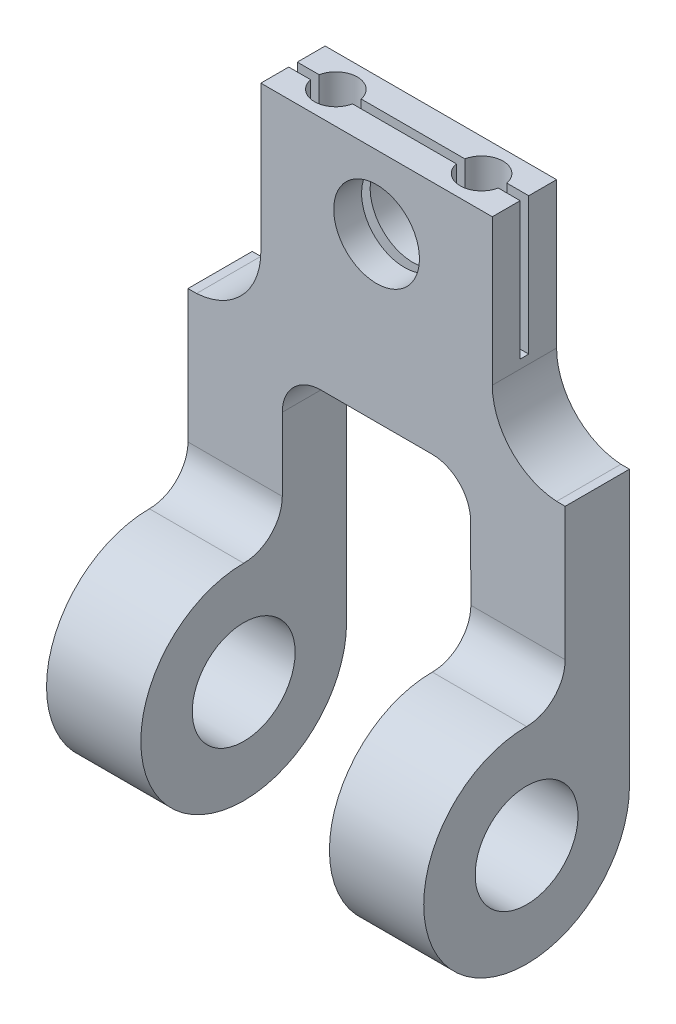
ISO-10303-21;
HEADER;
FILE_DESCRIPTION(('STEP AP214'),'2;1');
FILE_NAME('part.step','',(''),(''),'','','');
FILE_SCHEMA(('AUTOMOTIVE_DESIGN { 1 0 10303 214 1 1 1 1 }'));
ENDSEC;
DATA;
#1=APPLICATION_CONTEXT('core data for automotive mechanical design processes');
#2=APPLICATION_PROTOCOL_DEFINITION('international standard','automotive_design',2000,#1);
#3=PRODUCT_CONTEXT('',#1,'mechanical');
#4=PRODUCT('Part','Part','',(#3));
#5=PRODUCT_RELATED_PRODUCT_CATEGORY('part','',(#4));
#6=PRODUCT_DEFINITION_FORMATION('','',#4);
#7=PRODUCT_DEFINITION_CONTEXT('part definition',#1,'design');
#8=PRODUCT_DEFINITION('design','',#6,#7);
#9=PRODUCT_DEFINITION_SHAPE('','',#8);
#10=(LENGTH_UNIT() NAMED_UNIT(*) SI_UNIT(.MILLI.,.METRE.));
#11=(NAMED_UNIT(*) PLANE_ANGLE_UNIT() SI_UNIT($,.RADIAN.));
#12=(NAMED_UNIT(*) SI_UNIT($,.STERADIAN.) SOLID_ANGLE_UNIT());
#13=UNCERTAINTY_MEASURE_WITH_UNIT(LENGTH_MEASURE(1.E-05),#10,'distance_accuracy_value','');
#14=(GEOMETRIC_REPRESENTATION_CONTEXT(3) GLOBAL_UNCERTAINTY_ASSIGNED_CONTEXT((#13)) GLOBAL_UNIT_ASSIGNED_CONTEXT((#10,
#11,#12)) REPRESENTATION_CONTEXT('',''));
#15=CARTESIAN_POINT('',(0.,0.,0.));
#16=DIRECTION('',(0.,0.,1.));
#17=DIRECTION('',(1.,0.,0.));
#18=AXIS2_PLACEMENT_3D('',#15,#16,#17);
#19=CARTESIAN_POINT('',(88.,114.000000000021,-17.5));
#20=DIRECTION('',(0.,0.,-1.));
#21=DIRECTION('',(0.,1.,0.));
#22=AXIS2_PLACEMENT_3D('',#19,#20,#21);
#23=PLANE('',#22);
#24=DIRECTION('',(-1.,0.,0.));
#25=VECTOR('',#24,1.);
#26=CARTESIAN_POINT('',(88.,82.0000000000214,-17.5));
#27=LINE('',#26,#25);
#28=CARTESIAN_POINT('',(22.1010205144336,82.0000000000214,-17.5));
#29=VERTEX_POINT('',#28);
#30=CARTESIAN_POINT('',(17.,82.0000000000214,-17.5));
#31=VERTEX_POINT('',#30);
#32=EDGE_CURVE('E292',#29,#31,#27,.T.);
#33=ORIENTED_EDGE('',*,*,#32,.F.);
#34=DIRECTION('',(0.,1.,0.));
#35=VECTOR('',#34,1.);
#36=CARTESIAN_POINT('',(22.1010205144336,82.0000000000214,-17.5));
#37=LINE('',#36,#35);
#38=CARTESIAN_POINT('',(22.1010205144336,114.000000000021,-17.5));
#39=VERTEX_POINT('',#38);
#40=EDGE_CURVE('E341',#29,#39,#37,.T.);
#41=ORIENTED_EDGE('',*,*,#40,.T.);
#42=DIRECTION('',(-1.,0.,0.));
#43=VECTOR('',#42,1.);
#44=CARTESIAN_POINT('',(88.,114.000000000021,-17.5));
#45=LINE('',#44,#43);
#46=CARTESIAN_POINT('',(17.,114.000000000021,-17.5));
#47=VERTEX_POINT('',#46);
#48=EDGE_CURVE('E269',#39,#47,#45,.T.);
#49=ORIENTED_EDGE('',*,*,#48,.T.);
#50=DIRECTION('',(0.,-1.,0.));
#51=VECTOR('',#50,1.);
#52=CARTESIAN_POINT('',(17.,114.000000000021,-17.5));
#53=LINE('',#52,#51);
#54=EDGE_CURVE('E301',#47,#31,#53,.T.);
#55=ORIENTED_EDGE('',*,*,#54,.T.);
#56=EDGE_LOOP('',(#33,#41,#49,#55));
#57=FACE_BOUND('',#56,.T.);
#58=ADVANCED_FACE('F50',(#57),#23,.F.);
#59=CARTESIAN_POINT('',(44.,97.0000000000214,-17.5));
#60=DIRECTION('',(0.,0.,-1.));
#61=DIRECTION('',(0.,1.,0.));
#62=AXIS2_PLACEMENT_3D('',#59,#60,#61);
#63=CIRCLE('',#62,10.);
#64=CARTESIAN_POINT('',(44.,107.000000000021,-17.5));
#65=VERTEX_POINT('',#64);
#66=EDGE_CURVE('E601',#65,#65,#63,.F.);
#67=ORIENTED_EDGE('',*,*,#66,.F.);
#68=EDGE_LOOP('',(#67));
#69=FACE_BOUND('',#68,.T.);
#70=CARTESIAN_POINT('',(56.1010205144336,114.000000000021,-17.5));
#71=VERTEX_POINT('',#70);
#72=CARTESIAN_POINT('',(31.8989794855664,114.000000000021,-17.5));
#73=VERTEX_POINT('',#72);
#74=EDGE_CURVE('E273',#71,#73,#45,.T.);
#75=ORIENTED_EDGE('',*,*,#74,.T.);
#76=DIRECTION('',(0.,1.,0.));
#77=VECTOR('',#76,1.);
#78=CARTESIAN_POINT('',(31.8989794855664,82.0000000000214,-17.5));
#79=LINE('',#78,#77);
#80=CARTESIAN_POINT('',(31.8989794855664,82.0000000000214,-17.5));
#81=VERTEX_POINT('',#80);
#82=EDGE_CURVE('E317',#73,#81,#79,.F.);
#83=ORIENTED_EDGE('',*,*,#82,.T.);
#84=CARTESIAN_POINT('',(56.1010205144336,82.0000000000214,-17.5));
#85=VERTEX_POINT('',#84);
#86=EDGE_CURVE('E290',#85,#81,#27,.T.);
#87=ORIENTED_EDGE('',*,*,#86,.F.);
#88=DIRECTION('',(0.,1.,0.));
#89=VECTOR('',#88,1.);
#90=CARTESIAN_POINT('',(56.1010205144336,82.0000000000214,-17.5));
#91=LINE('',#90,#89);
#92=EDGE_CURVE('E319',#85,#71,#91,.T.);
#93=ORIENTED_EDGE('',*,*,#92,.T.);
#94=EDGE_LOOP('',(#75,#83,#87,#93));
#95=FACE_BOUND('',#94,.T.);
#96=ADVANCED_FACE('F320',(#69,#95),#23,.F.);
#97=CARTESIAN_POINT('',(88.,114.000000000021,-15.5));
#98=DIRECTION('',(0.,0.,1.));
#99=DIRECTION('',(0.,-1.,0.));
#100=AXIS2_PLACEMENT_3D('',#97,#98,#99);
#101=PLANE('',#100);
#102=CARTESIAN_POINT('',(44.,97.0000000000214,-15.5));
#103=DIRECTION('',(0.,0.,1.));
#104=DIRECTION('',(0.,-1.,0.));
#105=AXIS2_PLACEMENT_3D('',#102,#103,#104);
#106=CIRCLE('',#105,10.);
#107=CARTESIAN_POINT('',(44.,87.0000000000214,-15.5));
#108=VERTEX_POINT('',#107);
#109=EDGE_CURVE('E305',#108,#108,#106,.F.);
#110=ORIENTED_EDGE('',*,*,#109,.F.);
#111=EDGE_LOOP('',(#110));
#112=FACE_BOUND('',#111,.T.);
#113=DIRECTION('',(-1.,0.,0.));
#114=VECTOR('',#113,1.);
#115=CARTESIAN_POINT('',(88.,82.0000000000214,-15.5));
#116=LINE('',#115,#114);
#117=CARTESIAN_POINT('',(56.1010205144336,82.0000000000214,-15.5));
#118=VERTEX_POINT('',#117);
#119=CARTESIAN_POINT('',(31.8989794855664,82.0000000000214,-15.5));
#120=VERTEX_POINT('',#119);
#121=EDGE_CURVE('E283',#118,#120,#116,.T.);
#122=ORIENTED_EDGE('',*,*,#121,.T.);
#123=DIRECTION('',(0.,1.,0.));
#124=VECTOR('',#123,1.);
#125=CARTESIAN_POINT('',(31.8989794855664,82.0000000000214,-15.5));
#126=LINE('',#125,#124);
#127=CARTESIAN_POINT('',(31.8989794855664,114.000000000021,-15.5));
#128=VERTEX_POINT('',#127);
#129=EDGE_CURVE('E11',#120,#128,#126,.T.);
#130=ORIENTED_EDGE('',*,*,#129,.T.);
#131=DIRECTION('',(-1.,0.,0.));
#132=VECTOR('',#131,1.);
#133=CARTESIAN_POINT('',(88.,114.000000000021,-15.5));
#134=LINE('',#133,#132);
#135=CARTESIAN_POINT('',(56.1010205144336,114.000000000021,-15.5));
#136=VERTEX_POINT('',#135);
#137=EDGE_CURVE('E271',#136,#128,#134,.T.);
#138=ORIENTED_EDGE('',*,*,#137,.F.);
#139=DIRECTION('',(0.,1.,0.));
#140=VECTOR('',#139,1.);
#141=CARTESIAN_POINT('',(56.1010205144336,82.0000000000214,-15.5));
#142=LINE('',#141,#140);
#143=EDGE_CURVE('E252',#136,#118,#142,.F.);
#144=ORIENTED_EDGE('',*,*,#143,.T.);
#145=EDGE_LOOP('',(#122,#130,#138,#144));
#146=FACE_BOUND('',#145,.T.);
#147=ADVANCED_FACE('F352',(#112,#146),#101,.F.);
#148=CARTESIAN_POINT('',(71.,82.0000000000214,-15.5));
#149=VERTEX_POINT('',#148);
#150=CARTESIAN_POINT('',(65.8989794855663,82.0000000000214,-15.5));
#151=VERTEX_POINT('',#150);
#152=EDGE_CURVE('E262',#149,#151,#116,.T.);
#153=ORIENTED_EDGE('',*,*,#152,.T.);
#154=DIRECTION('',(0.,1.,0.));
#155=VECTOR('',#154,1.);
#156=CARTESIAN_POINT('',(65.8989794855663,82.0000000000214,-15.5));
#157=LINE('',#156,#155);
#158=CARTESIAN_POINT('',(65.8989794855663,114.000000000021,-15.5));
#159=VERTEX_POINT('',#158);
#160=EDGE_CURVE('E248',#151,#159,#157,.T.);
#161=ORIENTED_EDGE('',*,*,#160,.T.);
#162=CARTESIAN_POINT('',(71.,114.000000000021,-15.5));
#163=VERTEX_POINT('',#162);
#164=EDGE_CURVE('E265',#163,#159,#134,.T.);
#165=ORIENTED_EDGE('',*,*,#164,.F.);
#166=DIRECTION('',(0.,1.,0.));
#167=VECTOR('',#166,1.);
#168=CARTESIAN_POINT('',(71.,0.,-15.5));
#169=LINE('',#168,#167);
#170=EDGE_CURVE('E309',#149,#163,#169,.T.);
#171=ORIENTED_EDGE('',*,*,#170,.F.);
#172=EDGE_LOOP('',(#153,#161,#165,#171));
#173=FACE_BOUND('',#172,.T.);
#174=ADVANCED_FACE('F257',(#173),#101,.F.);
#175=CARTESIAN_POINT('',(0.,114.000000000021,-24.));
#176=DIRECTION('',(0.,-1.,0.));
#177=DIRECTION('',(0.,0.,-1.));
#178=AXIS2_PLACEMENT_3D('',#175,#176,#177);
#179=PLANE('',#178);
#180=ORIENTED_EDGE('',*,*,#48,.F.);
#181=CARTESIAN_POINT('',(27.,114.000000000021,-16.5));
#182=DIRECTION('',(0.,1.,0.));
#183=DIRECTION('',(0.,0.,1.));
#184=AXIS2_PLACEMENT_3D('',#181,#182,#183);
#185=CIRCLE('',#184,5.);
#186=EDGE_CURVE('E326',#73,#39,#185,.T.);
#187=ORIENTED_EDGE('',*,*,#186,.F.);
#188=ORIENTED_EDGE('',*,*,#74,.F.);
#189=CARTESIAN_POINT('',(61.,114.000000000021,-16.5));
#190=DIRECTION('',(0.,1.,0.));
#191=DIRECTION('',(0.,0.,1.));
#192=AXIS2_PLACEMENT_3D('',#189,#190,#191);
#193=CIRCLE('',#192,5.);
#194=CARTESIAN_POINT('',(65.8989794855663,114.000000000021,-17.5));
#195=VERTEX_POINT('',#194);
#196=EDGE_CURVE('E260',#195,#71,#193,.T.);
#197=ORIENTED_EDGE('',*,*,#196,.F.);
#198=CARTESIAN_POINT('',(71.,114.000000000021,-17.5));
#199=VERTEX_POINT('',#198);
#200=EDGE_CURVE('E277',#199,#195,#45,.T.);
#201=ORIENTED_EDGE('',*,*,#200,.F.);
#202=DIRECTION('',(0.,0.,1.));
#203=VECTOR('',#202,1.);
#204=CARTESIAN_POINT('',(71.,114.000000000021,-24.));
#205=LINE('',#204,#203);
#206=CARTESIAN_POINT('',(71.,114.000000000021,-24.));
#207=VERTEX_POINT('',#206);
#208=EDGE_CURVE('E541',#207,#199,#205,.T.);
#209=ORIENTED_EDGE('',*,*,#208,.F.);
#210=DIRECTION('',(1.,0.,0.));
#211=VECTOR('',#210,1.);
#212=CARTESIAN_POINT('',(0.,114.000000000021,-24.));
#213=LINE('',#212,#211);
#214=CARTESIAN_POINT('',(17.,114.000000000021,-24.));
#215=VERTEX_POINT('',#214);
#216=EDGE_CURVE('E488',#215,#207,#213,.T.);
#217=ORIENTED_EDGE('',*,*,#216,.F.);
#218=DIRECTION('',(0.,0.,1.));
#219=VECTOR('',#218,1.);
#220=CARTESIAN_POINT('',(17.,114.000000000021,-24.));
#221=LINE('',#220,#219);
#222=EDGE_CURVE('E538',#215,#47,#221,.T.);
#223=ORIENTED_EDGE('',*,*,#222,.T.);
#224=EDGE_LOOP('',(#180,#187,#188,#197,#201,#209,#217,#223));
#225=FACE_BOUND('',#224,.T.);
#226=ADVANCED_FACE('F324',(#225),#179,.F.);
#227=CARTESIAN_POINT('',(44.,97.0000000000214,-24.));
#228=DIRECTION('',(0.,0.,1.));
#229=DIRECTION('',(1.,0.,0.));
#230=AXIS2_PLACEMENT_3D('',#227,#228,#229);
#231=CYLINDRICAL_SURFACE('',#230,10.);
#232=ORIENTED_EDGE('',*,*,#66,.T.);
#233=EDGE_LOOP('',(#232));
#234=FACE_BOUND('',#233,.T.);
#235=CARTESIAN_POINT('',(44.,97.0000000000214,-24.));
#236=DIRECTION('',(0.,0.,1.));
#237=DIRECTION('',(1.,0.,0.));
#238=AXIS2_PLACEMENT_3D('',#235,#236,#237);
#239=CIRCLE('',#238,10.);
#240=CARTESIAN_POINT('',(54.,97.0000000000214,-24.));
#241=VERTEX_POINT('',#240);
#242=EDGE_CURVE('E474',#241,#241,#239,.T.);
#243=ORIENTED_EDGE('',*,*,#242,.F.);
#244=EDGE_LOOP('',(#243));
#245=FACE_BOUND('',#244,.T.);
#246=ADVANCED_FACE('F387',(#234,#245),#231,.F.);
#247=CARTESIAN_POINT('',(87.,79.9687194226927,-24.));
#248=DIRECTION('',(0.,0.,1.));
#249=DIRECTION('',(1.,0.,0.));
#250=AXIS2_PLACEMENT_3D('',#247,#248,#249);
#251=CYLINDRICAL_SURFACE('',#250,16.);
#252=DIRECTION('',(0.,0.,1.));
#253=VECTOR('',#252,1.);
#254=CARTESIAN_POINT('',(85.9999999999999,64.0000000000214,-24.));
#255=LINE('',#254,#253);
#256=CARTESIAN_POINT('',(85.9999999999999,64.0000000000214,-24.0000000000009));
#257=VERTEX_POINT('',#256);
#258=CARTESIAN_POINT('',(85.9999999999999,64.0000000000214,-9.00000000001455));
#259=VERTEX_POINT('',#258);
#260=EDGE_CURVE('E506',#257,#259,#255,.T.);
#261=ORIENTED_EDGE('',*,*,#260,.F.);
#262=CARTESIAN_POINT('',(87.,79.9687194226927,-24.));
#263=DIRECTION('',(0.,0.,1.));
#264=DIRECTION('',(1.,0.,0.));
#265=AXIS2_PLACEMENT_3D('',#262,#263,#264);
#266=CIRCLE('',#265,16.);
#267=CARTESIAN_POINT('',(71.,79.9687194226927,-24.));
#268=VERTEX_POINT('',#267);
#269=EDGE_CURVE('E476',#268,#257,#266,.T.);
#270=ORIENTED_EDGE('',*,*,#269,.F.);
#271=DIRECTION('',(0.,0.,1.));
#272=VECTOR('',#271,1.);
#273=CARTESIAN_POINT('',(71.,79.9687194226927,-24.));
#274=LINE('',#273,#272);
#275=CARTESIAN_POINT('',(71.,79.9687194226927,-9.00000000000001));
#276=VERTEX_POINT('',#275);
#277=EDGE_CURVE('E542',#268,#276,#274,.T.);
#278=ORIENTED_EDGE('',*,*,#277,.T.);
#279=CARTESIAN_POINT('',(87.,79.9687194226927,-9.00000000000001));
#280=DIRECTION('',(0.,0.,1.));
#281=DIRECTION('',(1.,0.,0.));
#282=AXIS2_PLACEMENT_3D('',#279,#280,#281);
#283=CIRCLE('',#282,16.);
#284=EDGE_CURVE('E521',#276,#259,#283,.T.);
#285=ORIENTED_EDGE('',*,*,#284,.T.);
#286=EDGE_LOOP('',(#261,#270,#278,#285));
#287=FACE_BOUND('',#286,.T.);
#288=ADVANCED_FACE('F423',(#287),#251,.F.);
#289=CARTESIAN_POINT('',(22.,64.,-24.));
#290=DIRECTION('',(0.,-1.,0.));
#291=DIRECTION('',(0.,0.,-1.));
#292=AXIS2_PLACEMENT_3D('',#289,#290,#291);
#293=PLANE('',#292);
#294=DIRECTION('',(0.,0.,1.));
#295=VECTOR('',#294,1.);
#296=CARTESIAN_POINT('',(2.0000611622042,64.,-24.));
#297=LINE('',#296,#295);
#298=CARTESIAN_POINT('',(2.0000611622042,64.,-24.));
#299=VERTEX_POINT('',#298);
#300=CARTESIAN_POINT('',(2.0000611622042,64.,-9.00000000000001));
#301=VERTEX_POINT('',#300);
#302=EDGE_CURVE('E540',#299,#301,#297,.T.);
#303=ORIENTED_EDGE('',*,*,#302,.F.);
#304=DIRECTION('',(-1.,0.,0.));
#305=VECTOR('',#304,1.);
#306=CARTESIAN_POINT('',(22.,64.,-24.));
#307=LINE('',#306,#305);
#308=CARTESIAN_POINT('',(0.,64.,-24.));
#309=VERTEX_POINT('',#308);
#310=EDGE_CURVE('E600',#299,#309,#307,.T.);
#311=ORIENTED_EDGE('',*,*,#310,.T.);
#312=DIRECTION('',(0.,0.,1.));
#313=VECTOR('',#312,1.);
#314=CARTESIAN_POINT('',(0.,64.,-24.));
#315=LINE('',#314,#313);
#316=CARTESIAN_POINT('',(0.,64.,-9.00000000000001));
#317=VERTEX_POINT('',#316);
#318=EDGE_CURVE('E585',#309,#317,#315,.T.);
#319=ORIENTED_EDGE('',*,*,#318,.T.);
#320=DIRECTION('',(-1.,0.,0.));
#321=VECTOR('',#320,1.);
#322=CARTESIAN_POINT('',(22.,64.,-9.00000000000001));
#323=LINE('',#322,#321);
#324=EDGE_CURVE('E594',#301,#317,#323,.T.);
#325=ORIENTED_EDGE('',*,*,#324,.F.);
#326=EDGE_LOOP('',(#303,#311,#319,#325));
#327=FACE_BOUND('',#326,.T.);
#328=ADVANCED_FACE('F424',(#327),#293,.F.);
#329=CARTESIAN_POINT('',(22.,0.,0.));
#330=DIRECTION('',(1.,0.,0.));
#331=DIRECTION('',(0.,0.,-1.));
#332=AXIS2_PLACEMENT_3D('',#329,#330,#331);
#333=PLANE('',#332);
#334=DIRECTION('',(0.,1.,0.));
#335=VECTOR('',#334,1.);
#336=CARTESIAN_POINT('',(22.,0.,-24.));
#337=LINE('',#336,#335);
#338=CARTESIAN_POINT('',(22.,0.,-24.));
#339=VERTEX_POINT('',#338);
#340=CARTESIAN_POINT('',(22.,50.0000000000213,-24.));
#341=VERTEX_POINT('',#340);
#342=EDGE_CURVE('E574',#339,#341,#337,.T.);
#343=ORIENTED_EDGE('',*,*,#342,.T.);
#344=DIRECTION('',(0.,0.,1.));
#345=VECTOR('',#344,1.);
#346=CARTESIAN_POINT('',(22.,50.0000000000213,-24.));
#347=LINE('',#346,#345);
#348=CARTESIAN_POINT('',(22.,50.0000000000213,-9.00000000000001));
#349=VERTEX_POINT('',#348);
#350=EDGE_CURVE('E503',#341,#349,#347,.T.);
#351=ORIENTED_EDGE('',*,*,#350,.T.);
#352=DIRECTION('',(0.,-1.,0.));
#353=VECTOR('',#352,1.);
#354=CARTESIAN_POINT('',(22.,64.,-9.00000000000001));
#355=LINE('',#354,#353);
#356=CARTESIAN_POINT('',(22.,33.,-9.00000000000001));
#357=VERTEX_POINT('',#356);
#358=EDGE_CURVE('E571',#349,#357,#355,.T.);
#359=ORIENTED_EDGE('',*,*,#358,.T.);
#360=CARTESIAN_POINT('',(22.,33.,0.));
#361=DIRECTION('',(-1.,0.,0.));
#362=DIRECTION('',(0.,0.,-1.));
#363=AXIS2_PLACEMENT_3D('',#360,#361,#362);
#364=CIRCLE('',#363,9.);
#365=CARTESIAN_POINT('',(22.,24.,0.));
#366=VERTEX_POINT('',#365);
#367=EDGE_CURVE('E577',#357,#366,#364,.T.);
#368=ORIENTED_EDGE('',*,*,#367,.T.);
#369=CARTESIAN_POINT('',(22.,0.,0.));
#370=DIRECTION('',(1.,0.,0.));
#371=DIRECTION('',(0.,0.,-1.));
#372=AXIS2_PLACEMENT_3D('',#369,#370,#371);
#373=CIRCLE('',#372,24.);
#374=EDGE_CURVE('E569',#366,#339,#373,.T.);
#375=ORIENTED_EDGE('',*,*,#374,.T.);
#376=EDGE_LOOP('',(#343,#351,#359,#368,#375));
#377=FACE_BOUND('',#376,.T.);
#378=CARTESIAN_POINT('',(22.,0.,0.));
#379=DIRECTION('',(1.,0.,0.));
#380=DIRECTION('',(0.,0.,-1.));
#381=AXIS2_PLACEMENT_3D('',#378,#379,#380);
#382=CIRCLE('',#381,12.);
#383=CARTESIAN_POINT('',(22.,0.,-12.));
#384=VERTEX_POINT('',#383);
#385=EDGE_CURVE('E564',#384,#384,#382,.T.);
#386=ORIENTED_EDGE('',*,*,#385,.F.);
#387=EDGE_LOOP('',(#386));
#388=FACE_BOUND('',#387,.T.);
#389=ADVANCED_FACE('F447',(#377,#388),#333,.T.);
#390=CARTESIAN_POINT('',(0.,0.,0.));
#391=DIRECTION('',(1.,0.,0.));
#392=DIRECTION('',(0.,0.,-1.));
#393=AXIS2_PLACEMENT_3D('',#390,#391,#392);
#394=PLANE('',#393);
#395=CARTESIAN_POINT('',(0.,33.,0.));
#396=DIRECTION('',(-1.,0.,0.));
#397=DIRECTION('',(0.,0.,-1.));
#398=AXIS2_PLACEMENT_3D('',#395,#396,#397);
#399=CIRCLE('',#398,9.);
#400=CARTESIAN_POINT('',(0.,33.,-9.00000000000001));
#401=VERTEX_POINT('',#400);
#402=CARTESIAN_POINT('',(0.,24.,0.));
#403=VERTEX_POINT('',#402);
#404=EDGE_CURVE('E572',#401,#403,#399,.T.);
#405=ORIENTED_EDGE('',*,*,#404,.F.);
#406=DIRECTION('',(0.,-1.,0.));
#407=VECTOR('',#406,1.);
#408=CARTESIAN_POINT('',(0.,64.,-9.00000000000001));
#409=LINE('',#408,#407);
#410=EDGE_CURVE('E590',#317,#401,#409,.T.);
#411=ORIENTED_EDGE('',*,*,#410,.F.);
#412=ORIENTED_EDGE('',*,*,#318,.F.);
#413=DIRECTION('',(0.,1.,0.));
#414=VECTOR('',#413,1.);
#415=CARTESIAN_POINT('',(0.,0.,-24.));
#416=LINE('',#415,#414);
#417=CARTESIAN_POINT('',(0.,0.,-24.));
#418=VERTEX_POINT('',#417);
#419=EDGE_CURVE('E582',#418,#309,#416,.T.);
#420=ORIENTED_EDGE('',*,*,#419,.F.);
#421=CARTESIAN_POINT('',(0.,0.,0.));
#422=DIRECTION('',(1.,0.,0.));
#423=DIRECTION('',(0.,0.,-1.));
#424=AXIS2_PLACEMENT_3D('',#421,#422,#423);
#425=CIRCLE('',#424,24.);
#426=EDGE_CURVE('E567',#403,#418,#425,.T.);
#427=ORIENTED_EDGE('',*,*,#426,.F.);
#428=EDGE_LOOP('',(#405,#411,#412,#420,#427));
#429=FACE_BOUND('',#428,.T.);
#430=CARTESIAN_POINT('',(0.,0.,0.));
#431=DIRECTION('',(1.,0.,0.));
#432=DIRECTION('',(0.,0.,-1.));
#433=AXIS2_PLACEMENT_3D('',#430,#431,#432);
#434=CIRCLE('',#433,12.);
#435=CARTESIAN_POINT('',(0.,0.,-12.));
#436=VERTEX_POINT('',#435);
#437=EDGE_CURVE('E562',#436,#436,#434,.T.);
#438=ORIENTED_EDGE('',*,*,#437,.T.);
#439=EDGE_LOOP('',(#438));
#440=FACE_BOUND('',#439,.T.);
#441=ADVANCED_FACE('F451',(#429,#440),#394,.F.);
#442=CARTESIAN_POINT('',(22.,0.,0.));
#443=DIRECTION('',(-1.,0.,0.));
#444=DIRECTION('',(0.,0.,1.));
#445=AXIS2_PLACEMENT_3D('',#442,#443,#444);
#446=CYLINDRICAL_SURFACE('',#445,24.);
#447=ORIENTED_EDGE('',*,*,#426,.T.);
#448=DIRECTION('',(-1.,0.,0.));
#449=VECTOR('',#448,1.);
#450=CARTESIAN_POINT('',(22.,0.,-24.));
#451=LINE('',#450,#449);
#452=EDGE_CURVE('E357',#339,#418,#451,.T.);
#453=ORIENTED_EDGE('',*,*,#452,.F.);
#454=ORIENTED_EDGE('',*,*,#374,.F.);
#455=DIRECTION('',(-1.,0.,0.));
#456=VECTOR('',#455,1.);
#457=CARTESIAN_POINT('',(22.,24.,0.));
#458=LINE('',#457,#456);
#459=EDGE_CURVE('E578',#366,#403,#458,.T.);
#460=ORIENTED_EDGE('',*,*,#459,.T.);
#461=EDGE_LOOP('',(#447,#453,#454,#460));
#462=FACE_BOUND('',#461,.T.);
#463=ADVANCED_FACE('F47',(#462),#446,.T.);
#464=CARTESIAN_POINT('',(22.,0.,-24.));
#465=DIRECTION('',(0.,0.,1.));
#466=DIRECTION('',(1.,0.,0.));
#467=AXIS2_PLACEMENT_3D('',#464,#465,#466);
#468=PLANE('',#467);
#469=ORIENTED_EDGE('',*,*,#242,.T.);
#470=EDGE_LOOP('',(#469));
#471=FACE_BOUND('',#470,.T.);
#472=ORIENTED_EDGE('',*,*,#269,.T.);
#473=DIRECTION('',(1.,0.,0.));
#474=VECTOR('',#473,1.);
#475=CARTESIAN_POINT('',(66.,64.0000000000214,-24.0000000000009));
#476=LINE('',#475,#474);
#477=CARTESIAN_POINT('',(88.,64.0000000000214,-24.0000000000009));
#478=VERTEX_POINT('',#477);
#479=EDGE_CURVE('E479',#257,#478,#476,.T.);
#480=ORIENTED_EDGE('',*,*,#479,.T.);
#481=DIRECTION('',(0.,1.,0.));
#482=VECTOR('',#481,1.);
#483=CARTESIAN_POINT('',(88.,0.,-24.));
#484=LINE('',#483,#482);
#485=CARTESIAN_POINT('',(88.,0.,-24.));
#486=VERTEX_POINT('',#485);
#487=EDGE_CURVE('E486',#486,#478,#484,.T.);
#488=ORIENTED_EDGE('',*,*,#487,.F.);
#489=DIRECTION('',(1.,0.,0.));
#490=VECTOR('',#489,1.);
#491=CARTESIAN_POINT('',(66.,0.,-24.));
#492=LINE('',#491,#490);
#493=CARTESIAN_POINT('',(66.,0.,-24.));
#494=VERTEX_POINT('',#493);
#495=EDGE_CURVE('E633',#494,#486,#492,.T.);
#496=ORIENTED_EDGE('',*,*,#495,.F.);
#497=DIRECTION('',(0.,-1.,0.));
#498=VECTOR('',#497,1.);
#499=CARTESIAN_POINT('',(66.,-291531.6,-24.0000000000009));
#500=LINE('',#499,#498);
#501=CARTESIAN_POINT('',(66.,33.0000000000155,-24.0000000000009));
#502=VERTEX_POINT('',#501);
#503=EDGE_CURVE('E621',#502,#494,#500,.T.);
#504=ORIENTED_EDGE('',*,*,#503,.F.);
#505=DIRECTION('',(0.00411668113619379,-0.999991526432311,0.));
#506=VECTOR('',#505,1.);
#507=CARTESIAN_POINT('',(66.1347308201602,0.272257905810401,-24.));
#508=LINE('',#507,#506);
#509=CARTESIAN_POINT('',(65.9298633028044,50.0370501302471,-24.));
#510=VERTEX_POINT('',#509);
#511=EDGE_CURVE('E491',#510,#502,#508,.T.);
#512=ORIENTED_EDGE('',*,*,#511,.F.);
#513=CARTESIAN_POINT('',(56.9299395649136,50.0000000000214,-24.));
#514=DIRECTION('',(0.,0.,1.));
#515=DIRECTION('',(1.,0.,0.));
#516=AXIS2_PLACEMENT_3D('',#513,#514,#515);
#517=CIRCLE('',#516,9.);
#518=CARTESIAN_POINT('',(56.9299395649136,59.0000000000214,-24.));
#519=VERTEX_POINT('',#518);
#520=EDGE_CURVE('E646',#519,#510,#517,.F.);
#521=ORIENTED_EDGE('',*,*,#520,.F.);
#522=DIRECTION('',(1.,0.,0.));
#523=VECTOR('',#522,1.);
#524=CARTESIAN_POINT('',(0.,59.0000000000214,-24.));
#525=LINE('',#524,#523);
#526=CARTESIAN_POINT('',(31.0000000000001,59.0000000000214,-24.));
#527=VERTEX_POINT('',#526);
#528=EDGE_CURVE('E641',#527,#519,#525,.T.);
#529=ORIENTED_EDGE('',*,*,#528,.F.);
#530=CARTESIAN_POINT('',(31.,50.0000000000214,-24.));
#531=DIRECTION('',(0.,0.,1.));
#532=DIRECTION('',(1.,0.,0.));
#533=AXIS2_PLACEMENT_3D('',#530,#531,#532);
#534=CIRCLE('',#533,9.);
#535=EDGE_CURVE('E531',#341,#527,#534,.F.);
#536=ORIENTED_EDGE('',*,*,#535,.F.);
#537=ORIENTED_EDGE('',*,*,#342,.F.);
#538=ORIENTED_EDGE('',*,*,#452,.T.);
#539=ORIENTED_EDGE('',*,*,#419,.T.);
#540=ORIENTED_EDGE('',*,*,#310,.F.);
#541=CARTESIAN_POINT('',(1.00003058110215,79.968717507579,-24.));
#542=DIRECTION('',(0.,0.,1.));
#543=DIRECTION('',(1.,0.,0.));
#544=AXIS2_PLACEMENT_3D('',#541,#542,#543);
#545=CIRCLE('',#544,16.);
#546=CARTESIAN_POINT('',(17.,80.0000000000214,-24.));
#547=VERTEX_POINT('',#546);
#548=EDGE_CURVE('E496',#299,#547,#545,.T.);
#549=ORIENTED_EDGE('',*,*,#548,.T.);
#550=DIRECTION('',(0.,-1.,0.));
#551=VECTOR('',#550,1.);
#552=CARTESIAN_POINT('',(17.,0.,-24.));
#553=LINE('',#552,#551);
#554=EDGE_CURVE('E497',#215,#547,#553,.T.);
#555=ORIENTED_EDGE('',*,*,#554,.F.);
#556=ORIENTED_EDGE('',*,*,#216,.T.);
#557=DIRECTION('',(0.,-1.,0.));
#558=VECTOR('',#557,1.);
#559=CARTESIAN_POINT('',(71.,0.,-24.));
#560=LINE('',#559,#558);
#561=EDGE_CURVE('E485',#207,#268,#560,.T.);
#562=ORIENTED_EDGE('',*,*,#561,.T.);
#563=EDGE_LOOP('',(#472,#480,#488,#496,#504,#512,#521,#529,#536,#537,#538,#539,#540,#549,#555,
#556,#562));
#564=FACE_BOUND('',#563,.T.);
#565=ADVANCED_FACE('F464',(#471,#564),#468,.F.);
#566=CARTESIAN_POINT('',(22.,64.,-9.00000000000001));
#567=DIRECTION('',(0.,0.,-1.));
#568=DIRECTION('',(-1.,0.,0.));
#569=AXIS2_PLACEMENT_3D('',#566,#567,#568);
#570=PLANE('',#569);
#571=CARTESIAN_POINT('',(44.,97.0000000000214,-9.00000000000001));
#572=DIRECTION('',(0.,0.,1.));
#573=DIRECTION('',(1.,0.,0.));
#574=AXIS2_PLACEMENT_3D('',#571,#572,#573);
#575=CIRCLE('',#574,10.);
#576=CARTESIAN_POINT('',(54.,97.0000000000214,-9.00000000000001));
#577=VERTEX_POINT('',#576);
#578=EDGE_CURVE('E610',#577,#577,#575,.T.);
#579=ORIENTED_EDGE('',*,*,#578,.F.);
#580=EDGE_LOOP('',(#579));
#581=FACE_BOUND('',#580,.T.);
#582=DIRECTION('',(0.,1.,0.));
#583=VECTOR('',#582,1.);
#584=CARTESIAN_POINT('',(88.,0.,-9.00000000000001));
#585=LINE('',#584,#583);
#586=CARTESIAN_POINT('',(88.,33.0000000000155,-9.00000000001455));
#587=VERTEX_POINT('',#586);
#588=CARTESIAN_POINT('',(88.,64.0000000000214,-9.00000000000001));
#589=VERTEX_POINT('',#588);
#590=EDGE_CURVE('E517',#587,#589,#585,.T.);
#591=ORIENTED_EDGE('',*,*,#590,.T.);
#592=DIRECTION('',(1.,0.,0.));
#593=VECTOR('',#592,1.);
#594=CARTESIAN_POINT('',(66.,64.0000000000214,-9.00000000001455));
#595=LINE('',#594,#593);
#596=EDGE_CURVE('E636',#259,#589,#595,.T.);
#597=ORIENTED_EDGE('',*,*,#596,.F.);
#598=ORIENTED_EDGE('',*,*,#284,.F.);
#599=DIRECTION('',(0.,-1.,0.));
#600=VECTOR('',#599,1.);
#601=CARTESIAN_POINT('',(71.,0.,-9.00000000000001));
#602=LINE('',#601,#600);
#603=CARTESIAN_POINT('',(71.,114.000000000021,-9.00000000000001));
#604=VERTEX_POINT('',#603);
#605=EDGE_CURVE('E523',#604,#276,#602,.T.);
#606=ORIENTED_EDGE('',*,*,#605,.F.);
#607=DIRECTION('',(1.,0.,0.));
#608=VECTOR('',#607,1.);
#609=CARTESIAN_POINT('',(0.,114.000000000021,-9.00000000000001));
#610=LINE('',#609,#608);
#611=CARTESIAN_POINT('',(17.,114.000000000021,-9.00000000000001));
#612=VERTEX_POINT('',#611);
#613=EDGE_CURVE('E528',#612,#604,#610,.T.);
#614=ORIENTED_EDGE('',*,*,#613,.F.);
#615=DIRECTION('',(0.,-1.,0.));
#616=VECTOR('',#615,1.);
#617=CARTESIAN_POINT('',(17.,0.,-9.00000000000001));
#618=LINE('',#617,#616);
#619=CARTESIAN_POINT('',(17.,80.0000000000214,-9.00000000000001));
#620=VERTEX_POINT('',#619);
#621=EDGE_CURVE('E526',#612,#620,#618,.T.);
#622=ORIENTED_EDGE('',*,*,#621,.T.);
#623=CARTESIAN_POINT('',(1.00003058110215,79.968717507579,-9.00000000000001));
#624=DIRECTION('',(0.,0.,1.));
#625=DIRECTION('',(1.,0.,0.));
#626=AXIS2_PLACEMENT_3D('',#623,#624,#625);
#627=CIRCLE('',#626,16.);
#628=EDGE_CURVE('E533',#301,#620,#627,.T.);
#629=ORIENTED_EDGE('',*,*,#628,.F.);
#630=ORIENTED_EDGE('',*,*,#324,.T.);
#631=ORIENTED_EDGE('',*,*,#410,.T.);
#632=DIRECTION('',(-1.,0.,0.));
#633=VECTOR('',#632,1.);
#634=CARTESIAN_POINT('',(22.,33.,-9.00000000000001));
#635=LINE('',#634,#633);
#636=EDGE_CURVE('E595',#357,#401,#635,.T.);
#637=ORIENTED_EDGE('',*,*,#636,.F.);
#638=ORIENTED_EDGE('',*,*,#358,.F.);
#639=CARTESIAN_POINT('',(31.,50.0000000000214,-9.00000000000001));
#640=DIRECTION('',(0.,0.,1.));
#641=DIRECTION('',(1.,0.,0.));
#642=AXIS2_PLACEMENT_3D('',#639,#640,#641);
#643=CIRCLE('',#642,9.);
#644=CARTESIAN_POINT('',(31.0000000000001,59.0000000000214,-9.00000000000001));
#645=VERTEX_POINT('',#644);
#646=EDGE_CURVE('E504',#349,#645,#643,.F.);
#647=ORIENTED_EDGE('',*,*,#646,.T.);
#648=DIRECTION('',(1.,0.,0.));
#649=VECTOR('',#648,1.);
#650=CARTESIAN_POINT('',(0.,59.0000000000214,-9.00000000000001));
#651=LINE('',#650,#649);
#652=CARTESIAN_POINT('',(56.9299395649136,59.0000000000214,-9.00000000000001));
#653=VERTEX_POINT('',#652);
#654=EDGE_CURVE('E501',#645,#653,#651,.T.);
#655=ORIENTED_EDGE('',*,*,#654,.T.);
#656=CARTESIAN_POINT('',(56.9299395649136,50.0000000000214,-9.00000000000001));
#657=DIRECTION('',(0.,0.,1.));
#658=DIRECTION('',(1.,0.,0.));
#659=AXIS2_PLACEMENT_3D('',#656,#657,#658);
#660=CIRCLE('',#659,9.);
#661=CARTESIAN_POINT('',(65.9298633028044,50.0370501302471,-9.00000000000001));
#662=VERTEX_POINT('',#661);
#663=EDGE_CURVE('E508',#653,#662,#660,.F.);
#664=ORIENTED_EDGE('',*,*,#663,.T.);
#665=DIRECTION('',(0.00411668113619379,-0.999991526432311,0.));
#666=VECTOR('',#665,1.);
#667=CARTESIAN_POINT('',(66.1347308201602,0.272257905810401,-9.00000000000001));
#668=LINE('',#667,#666);
#669=CARTESIAN_POINT('',(66.,33.0000000000155,-9.00000000000001));
#670=VERTEX_POINT('',#669);
#671=EDGE_CURVE('E515',#662,#670,#668,.T.);
#672=ORIENTED_EDGE('',*,*,#671,.T.);
#673=DIRECTION('',(1.,0.,0.));
#674=VECTOR('',#673,1.);
#675=CARTESIAN_POINT('',(0.,33.0000000000155,-9.00000000000001));
#676=LINE('',#675,#674);
#677=EDGE_CURVE('E513',#670,#587,#676,.T.);
#678=ORIENTED_EDGE('',*,*,#677,.T.);
#679=EDGE_LOOP('',(#591,#597,#598,#606,#614,#622,#629,#630,#631,#637,#638,#647,#655,#664,#672,#678));
#680=FACE_BOUND('',#679,.T.);
#681=ADVANCED_FACE('F456',(#581,#680),#570,.F.);
#682=CARTESIAN_POINT('',(22.,33.,0.));
#683=DIRECTION('',(-1.,0.,0.));
#684=DIRECTION('',(0.,0.,1.));
#685=AXIS2_PLACEMENT_3D('',#682,#683,#684);
#686=CYLINDRICAL_SURFACE('',#685,9.);
#687=ORIENTED_EDGE('',*,*,#404,.T.);
#688=ORIENTED_EDGE('',*,*,#459,.F.);
#689=ORIENTED_EDGE('',*,*,#367,.F.);
#690=ORIENTED_EDGE('',*,*,#636,.T.);
#691=EDGE_LOOP('',(#687,#688,#689,#690));
#692=FACE_BOUND('',#691,.T.);
#693=ADVANCED_FACE('F448',(#692),#686,.F.);
#694=CARTESIAN_POINT('',(22.,0.,0.));
#695=DIRECTION('',(-1.,0.,0.));
#696=DIRECTION('',(0.,0.,1.));
#697=AXIS2_PLACEMENT_3D('',#694,#695,#696);
#698=CYLINDRICAL_SURFACE('',#697,12.);
#699=ORIENTED_EDGE('',*,*,#385,.T.);
#700=EDGE_LOOP('',(#699));
#701=FACE_BOUND('',#700,.T.);
#702=ORIENTED_EDGE('',*,*,#437,.F.);
#703=EDGE_LOOP('',(#702));
#704=FACE_BOUND('',#703,.T.);
#705=ADVANCED_FACE('F406',(#701,#704),#698,.F.);
#706=CARTESIAN_POINT('',(1.00003058110215,79.968717507579,-24.));
#707=DIRECTION('',(0.,0.,1.));
#708=DIRECTION('',(1.,0.,0.));
#709=AXIS2_PLACEMENT_3D('',#706,#707,#708);
#710=CYLINDRICAL_SURFACE('',#709,16.);
#711=ORIENTED_EDGE('',*,*,#548,.F.);
#712=ORIENTED_EDGE('',*,*,#302,.T.);
#713=ORIENTED_EDGE('',*,*,#628,.T.);
#714=DIRECTION('',(0.,0.,1.));
#715=VECTOR('',#714,1.);
#716=CARTESIAN_POINT('',(17.,80.0000000000214,-24.));
#717=LINE('',#716,#715);
#718=EDGE_CURVE('E534',#547,#620,#717,.T.);
#719=ORIENTED_EDGE('',*,*,#718,.F.);
#720=EDGE_LOOP('',(#711,#712,#713,#719));
#721=FACE_BOUND('',#720,.T.);
#722=ADVANCED_FACE('F409',(#721),#710,.F.);
#723=CARTESIAN_POINT('',(17.,0.,-24.));
#724=DIRECTION('',(-1.,0.,0.));
#725=DIRECTION('',(0.,0.,1.));
#726=AXIS2_PLACEMENT_3D('',#723,#724,#725);
#727=PLANE('',#726);
#728=ORIENTED_EDGE('',*,*,#54,.F.);
#729=ORIENTED_EDGE('',*,*,#222,.F.);
#730=ORIENTED_EDGE('',*,*,#554,.T.);
#731=ORIENTED_EDGE('',*,*,#718,.T.);
#732=ORIENTED_EDGE('',*,*,#621,.F.);
#733=CARTESIAN_POINT('',(17.,114.000000000021,-15.5));
#734=VERTEX_POINT('',#733);
#735=EDGE_CURVE('E539',#734,#612,#221,.T.);
#736=ORIENTED_EDGE('',*,*,#735,.F.);
#737=DIRECTION('',(0.,1.,0.));
#738=VECTOR('',#737,1.);
#739=CARTESIAN_POINT('',(17.,114.000000000021,-15.5));
#740=LINE('',#739,#738);
#741=CARTESIAN_POINT('',(17.,82.0000000000214,-15.5));
#742=VERTEX_POINT('',#741);
#743=EDGE_CURVE('E294',#742,#734,#740,.T.);
#744=ORIENTED_EDGE('',*,*,#743,.F.);
#745=DIRECTION('',(0.,0.,1.));
#746=VECTOR('',#745,1.);
#747=CARTESIAN_POINT('',(17.,82.0000000000214,-17.5));
#748=LINE('',#747,#746);
#749=EDGE_CURVE('E299',#31,#742,#748,.T.);
#750=ORIENTED_EDGE('',*,*,#749,.F.);
#751=EDGE_LOOP('',(#728,#729,#730,#731,#732,#736,#744,#750));
#752=FACE_BOUND('',#751,.T.);
#753=ADVANCED_FACE('F347',(#752),#727,.T.);
#754=ORIENTED_EDGE('',*,*,#137,.T.);
#755=CARTESIAN_POINT('',(22.1010205144336,114.000000000021,-15.5));
#756=VERTEX_POINT('',#755);
#757=EDGE_CURVE('E332',#756,#128,#185,.T.);
#758=ORIENTED_EDGE('',*,*,#757,.F.);
#759=EDGE_CURVE('E272',#756,#734,#134,.T.);
#760=ORIENTED_EDGE('',*,*,#759,.T.);
#761=ORIENTED_EDGE('',*,*,#735,.T.);
#762=ORIENTED_EDGE('',*,*,#613,.T.);
#763=EDGE_CURVE('E267',#163,#604,#205,.T.);
#764=ORIENTED_EDGE('',*,*,#763,.F.);
#765=ORIENTED_EDGE('',*,*,#164,.T.);
#766=EDGE_CURVE('E246',#136,#159,#193,.T.);
#767=ORIENTED_EDGE('',*,*,#766,.F.);
#768=EDGE_LOOP('',(#754,#758,#760,#761,#762,#764,#765,#767));
#769=FACE_BOUND('',#768,.T.);
#770=ADVANCED_FACE('F270',(#769),#179,.F.);
#771=CARTESIAN_POINT('',(71.,0.,-24.));
#772=DIRECTION('',(-1.,0.,0.));
#773=DIRECTION('',(0.,0.,1.));
#774=AXIS2_PLACEMENT_3D('',#771,#772,#773);
#775=PLANE('',#774);
#776=ORIENTED_EDGE('',*,*,#208,.T.);
#777=DIRECTION('',(0.,-1.,0.));
#778=VECTOR('',#777,1.);
#779=CARTESIAN_POINT('',(71.,0.,-17.5));
#780=LINE('',#779,#778);
#781=CARTESIAN_POINT('',(71.,82.0000000000214,-17.5));
#782=VERTEX_POINT('',#781);
#783=EDGE_CURVE('E602',#199,#782,#780,.T.);
#784=ORIENTED_EDGE('',*,*,#783,.T.);
#785=DIRECTION('',(0.,0.,1.));
#786=VECTOR('',#785,1.);
#787=CARTESIAN_POINT('',(71.,82.0000000000214,-24.));
#788=LINE('',#787,#786);
#789=EDGE_CURVE('E355',#782,#149,#788,.T.);
#790=ORIENTED_EDGE('',*,*,#789,.T.);
#791=ORIENTED_EDGE('',*,*,#170,.T.);
#792=ORIENTED_EDGE('',*,*,#763,.T.);
#793=ORIENTED_EDGE('',*,*,#605,.T.);
#794=ORIENTED_EDGE('',*,*,#277,.F.);
#795=ORIENTED_EDGE('',*,*,#561,.F.);
#796=EDGE_LOOP('',(#776,#784,#790,#791,#792,#793,#794,#795));
#797=FACE_BOUND('',#796,.T.);
#798=ADVANCED_FACE('F418',(#797),#775,.F.);
#799=CARTESIAN_POINT('',(88.,0.,-24.));
#800=DIRECTION('',(1.,0.,0.));
#801=DIRECTION('',(0.,0.,-1.));
#802=AXIS2_PLACEMENT_3D('',#799,#800,#801);
#803=PLANE('',#802);
#804=ORIENTED_EDGE('',*,*,#590,.F.);
#805=CARTESIAN_POINT('',(88.,33.,0.));
#806=DIRECTION('',(1.,0.,0.));
#807=DIRECTION('',(0.,0.,-1.));
#808=AXIS2_PLACEMENT_3D('',#805,#806,#807);
#809=CIRCLE('',#808,9.);
#810=CARTESIAN_POINT('',(88.,24.,0.));
#811=VERTEX_POINT('',#810);
#812=EDGE_CURVE('E617',#811,#587,#809,.T.);
#813=ORIENTED_EDGE('',*,*,#812,.F.);
#814=CARTESIAN_POINT('',(88.,0.,0.));
#815=DIRECTION('',(1.,0.,0.));
#816=DIRECTION('',(0.,0.,-1.));
#817=AXIS2_PLACEMENT_3D('',#814,#815,#816);
#818=CIRCLE('',#817,24.);
#819=EDGE_CURVE('E624',#811,#486,#818,.T.);
#820=ORIENTED_EDGE('',*,*,#819,.T.);
#821=ORIENTED_EDGE('',*,*,#487,.T.);
#822=DIRECTION('',(0.,0.,1.));
#823=VECTOR('',#822,1.);
#824=CARTESIAN_POINT('',(88.,64.0000000000214,-24.));
#825=LINE('',#824,#823);
#826=EDGE_CURVE('E546',#478,#589,#825,.T.);
#827=ORIENTED_EDGE('',*,*,#826,.T.);
#828=EDGE_LOOP('',(#804,#813,#820,#821,#827));
#829=FACE_BOUND('',#828,.T.);
#830=CARTESIAN_POINT('',(88.,0.,0.));
#831=DIRECTION('',(1.,0.,0.));
#832=DIRECTION('',(0.,0.,-1.));
#833=AXIS2_PLACEMENT_3D('',#830,#831,#832);
#834=CIRCLE('',#833,12.);
#835=CARTESIAN_POINT('',(88.,0.,-12.));
#836=VERTEX_POINT('',#835);
#837=EDGE_CURVE('E613',#836,#836,#834,.T.);
#838=ORIENTED_EDGE('',*,*,#837,.F.);
#839=EDGE_LOOP('',(#838));
#840=FACE_BOUND('',#839,.T.);
#841=ADVANCED_FACE('F420',(#829,#840),#803,.T.);
#842=CARTESIAN_POINT('',(66.1347308201602,0.272257905810401,-24.));
#843=DIRECTION('',(-0.999991526432311,-0.00411668113619379,0.));
#844=DIRECTION('',(0.00411668113619379,-0.999991526432311,0.));
#845=AXIS2_PLACEMENT_3D('',#842,#843,#844);
#846=PLANE('',#845);
#847=ORIENTED_EDGE('',*,*,#671,.F.);
#848=DIRECTION('',(0.,0.,1.));
#849=VECTOR('',#848,1.);
#850=CARTESIAN_POINT('',(65.9298633028044,50.0370501302471,-24.));
#851=LINE('',#850,#849);
#852=EDGE_CURVE('E555',#510,#662,#851,.T.);
#853=ORIENTED_EDGE('',*,*,#852,.F.);
#854=ORIENTED_EDGE('',*,*,#511,.T.);
#855=DIRECTION('',(0.,0.,1.));
#856=VECTOR('',#855,1.);
#857=CARTESIAN_POINT('',(66.,33.0000000000155,-24.));
#858=LINE('',#857,#856);
#859=EDGE_CURVE('E548',#502,#670,#858,.T.);
#860=ORIENTED_EDGE('',*,*,#859,.T.);
#861=EDGE_LOOP('',(#847,#853,#854,#860));
#862=FACE_BOUND('',#861,.T.);
#863=ADVANCED_FACE('F428',(#862),#846,.T.);
#864=CARTESIAN_POINT('',(56.9299395649136,50.0000000000214,-24.));
#865=DIRECTION('',(0.,0.,1.));
#866=DIRECTION('',(1.,0.,0.));
#867=AXIS2_PLACEMENT_3D('',#864,#865,#866);
#868=CYLINDRICAL_SURFACE('',#867,9.);
#869=ORIENTED_EDGE('',*,*,#663,.F.);
#870=DIRECTION('',(0.,0.,1.));
#871=VECTOR('',#870,1.);
#872=CARTESIAN_POINT('',(56.9299395649136,59.0000000000214,-24.));
#873=LINE('',#872,#871);
#874=EDGE_CURVE('E551',#519,#653,#873,.T.);
#875=ORIENTED_EDGE('',*,*,#874,.F.);
#876=ORIENTED_EDGE('',*,*,#520,.T.);
#877=ORIENTED_EDGE('',*,*,#852,.T.);
#878=EDGE_LOOP('',(#869,#875,#876,#877));
#879=FACE_BOUND('',#878,.T.);
#880=ADVANCED_FACE('F435',(#879),#868,.F.);
#881=CARTESIAN_POINT('',(0.,59.0000000000214,-24.));
#882=DIRECTION('',(0.,-1.,0.));
#883=DIRECTION('',(0.,0.,-1.));
#884=AXIS2_PLACEMENT_3D('',#881,#882,#883);
#885=PLANE('',#884);
#886=ORIENTED_EDGE('',*,*,#654,.F.);
#887=DIRECTION('',(0.,0.,1.));
#888=VECTOR('',#887,1.);
#889=CARTESIAN_POINT('',(31.0000000000001,59.0000000000214,-24.));
#890=LINE('',#889,#888);
#891=EDGE_CURVE('E558',#527,#645,#890,.T.);
#892=ORIENTED_EDGE('',*,*,#891,.F.);
#893=ORIENTED_EDGE('',*,*,#528,.T.);
#894=ORIENTED_EDGE('',*,*,#874,.T.);
#895=EDGE_LOOP('',(#886,#892,#893,#894));
#896=FACE_BOUND('',#895,.T.);
#897=ADVANCED_FACE('F436',(#896),#885,.T.);
#898=CARTESIAN_POINT('',(31.,50.0000000000214,-24.));
#899=DIRECTION('',(0.,0.,1.));
#900=DIRECTION('',(1.,0.,0.));
#901=AXIS2_PLACEMENT_3D('',#898,#899,#900);
#902=CYLINDRICAL_SURFACE('',#901,9.);
#903=ORIENTED_EDGE('',*,*,#646,.F.);
#904=ORIENTED_EDGE('',*,*,#350,.F.);
#905=ORIENTED_EDGE('',*,*,#535,.T.);
#906=ORIENTED_EDGE('',*,*,#891,.T.);
#907=EDGE_LOOP('',(#903,#904,#905,#906));
#908=FACE_BOUND('',#907,.T.);
#909=ADVANCED_FACE('F393',(#908),#902,.F.);
#910=CARTESIAN_POINT('',(66.,0.,0.));
#911=DIRECTION('',(1.,0.,0.));
#912=DIRECTION('',(0.,0.,-1.));
#913=AXIS2_PLACEMENT_3D('',#910,#911,#912);
#914=CYLINDRICAL_SURFACE('',#913,12.);
#915=CARTESIAN_POINT('',(66.,0.,0.));
#916=DIRECTION('',(1.,0.,0.));
#917=DIRECTION('',(0.,0.,-1.));
#918=AXIS2_PLACEMENT_3D('',#915,#916,#917);
#919=CIRCLE('',#918,12.);
#920=CARTESIAN_POINT('',(66.,0.,-12.));
#921=VERTEX_POINT('',#920);
#922=EDGE_CURVE('E615',#921,#921,#919,.T.);
#923=ORIENTED_EDGE('',*,*,#922,.F.);
#924=EDGE_LOOP('',(#923));
#925=FACE_BOUND('',#924,.T.);
#926=ORIENTED_EDGE('',*,*,#837,.T.);
#927=EDGE_LOOP('',(#926));
#928=FACE_BOUND('',#927,.T.);
#929=ADVANCED_FACE('F390',(#925,#928),#914,.F.);
#930=CARTESIAN_POINT('',(66.,33.,0.));
#931=DIRECTION('',(1.,0.,0.));
#932=DIRECTION('',(0.,0.,-1.));
#933=AXIS2_PLACEMENT_3D('',#930,#931,#932);
#934=PLANE('',#933);
#935=ORIENTED_EDGE('',*,*,#859,.F.);
#936=ORIENTED_EDGE('',*,*,#503,.T.);
#937=CARTESIAN_POINT('',(66.,0.,0.));
#938=DIRECTION('',(1.,0.,0.));
#939=DIRECTION('',(0.,0.,-1.));
#940=AXIS2_PLACEMENT_3D('',#937,#938,#939);
#941=CIRCLE('',#940,24.);
#942=CARTESIAN_POINT('',(66.,24.,0.));
#943=VERTEX_POINT('',#942);
#944=EDGE_CURVE('E628',#943,#494,#941,.T.);
#945=ORIENTED_EDGE('',*,*,#944,.F.);
#946=CARTESIAN_POINT('',(66.,33.,0.));
#947=DIRECTION('',(1.,0.,0.));
#948=DIRECTION('',(0.,0.,-1.));
#949=AXIS2_PLACEMENT_3D('',#946,#947,#948);
#950=CIRCLE('',#949,9.);
#951=EDGE_CURVE('E620',#943,#670,#950,.T.);
#952=ORIENTED_EDGE('',*,*,#951,.T.);
#953=EDGE_LOOP('',(#935,#936,#945,#952));
#954=FACE_BOUND('',#953,.T.);
#955=ORIENTED_EDGE('',*,*,#922,.T.);
#956=EDGE_LOOP('',(#955));
#957=FACE_BOUND('',#956,.T.);
#958=ADVANCED_FACE('F388',(#954,#957),#934,.F.);
#959=CARTESIAN_POINT('',(66.,0.,0.));
#960=DIRECTION('',(1.,0.,0.));
#961=DIRECTION('',(0.,0.,-1.));
#962=AXIS2_PLACEMENT_3D('',#959,#960,#961);
#963=CYLINDRICAL_SURFACE('',#962,24.);
#964=ORIENTED_EDGE('',*,*,#819,.F.);
#965=DIRECTION('',(1.,0.,0.));
#966=VECTOR('',#965,1.);
#967=CARTESIAN_POINT('',(66.,24.,0.));
#968=LINE('',#967,#966);
#969=EDGE_CURVE('E630',#943,#811,#968,.T.);
#970=ORIENTED_EDGE('',*,*,#969,.F.);
#971=ORIENTED_EDGE('',*,*,#944,.T.);
#972=ORIENTED_EDGE('',*,*,#495,.T.);
#973=EDGE_LOOP('',(#964,#970,#971,#972));
#974=FACE_BOUND('',#973,.T.);
#975=ADVANCED_FACE('F391',(#974),#963,.T.);
#976=CARTESIAN_POINT('',(66.,33.,0.));
#977=DIRECTION('',(1.,0.,0.));
#978=DIRECTION('',(0.,0.,-1.));
#979=AXIS2_PLACEMENT_3D('',#976,#977,#978);
#980=CYLINDRICAL_SURFACE('',#979,9.);
#981=ORIENTED_EDGE('',*,*,#812,.T.);
#982=ORIENTED_EDGE('',*,*,#677,.F.);
#983=ORIENTED_EDGE('',*,*,#951,.F.);
#984=ORIENTED_EDGE('',*,*,#969,.T.);
#985=EDGE_LOOP('',(#981,#982,#983,#984));
#986=FACE_BOUND('',#985,.T.);
#987=ADVANCED_FACE('F398',(#986),#980,.F.);
#988=CARTESIAN_POINT('',(66.,64.0000000000214,400000.));
#989=DIRECTION('',(0.,-1.,0.));
#990=DIRECTION('',(0.,0.,-1.));
#991=AXIS2_PLACEMENT_3D('',#988,#989,#990);
#992=PLANE('',#991);
#993=ORIENTED_EDGE('',*,*,#479,.F.);
#994=ORIENTED_EDGE('',*,*,#260,.T.);
#995=ORIENTED_EDGE('',*,*,#596,.T.);
#996=ORIENTED_EDGE('',*,*,#826,.F.);
#997=EDGE_LOOP('',(#993,#994,#995,#996));
#998=FACE_BOUND('',#997,.T.);
#999=ADVANCED_FACE('F383',(#998),#992,.F.);
#1000=ORIENTED_EDGE('',*,*,#109,.T.);
#1001=EDGE_LOOP('',(#1000));
#1002=FACE_BOUND('',#1001,.T.);
#1003=ORIENTED_EDGE('',*,*,#578,.T.);
#1004=EDGE_LOOP('',(#1003));
#1005=FACE_BOUND('',#1004,.T.);
#1006=ADVANCED_FACE('F381',(#1002,#1005),#231,.F.);
#1007=CARTESIAN_POINT('',(88.,82.0000000000214,-17.5));
#1008=DIRECTION('',(0.,-1.,0.));
#1009=DIRECTION('',(0.,0.,-1.));
#1010=AXIS2_PLACEMENT_3D('',#1007,#1008,#1009);
#1011=PLANE('',#1010);
#1012=CARTESIAN_POINT('',(22.1010205144336,82.0000000000214,-15.5));
#1013=VERTEX_POINT('',#1012);
#1014=EDGE_CURVE('E284',#1013,#742,#116,.T.);
#1015=ORIENTED_EDGE('',*,*,#1014,.F.);
#1016=CARTESIAN_POINT('',(27.,82.0000000000214,-16.5));
#1017=DIRECTION('',(0.,1.,0.));
#1018=DIRECTION('',(0.,0.,1.));
#1019=AXIS2_PLACEMENT_3D('',#1016,#1017,#1018);
#1020=CIRCLE('',#1019,5.);
#1021=EDGE_CURVE('E329',#1013,#120,#1020,.T.);
#1022=ORIENTED_EDGE('',*,*,#1021,.T.);
#1023=ORIENTED_EDGE('',*,*,#121,.F.);
#1024=CARTESIAN_POINT('',(61.,82.0000000000214,-16.5));
#1025=DIRECTION('',(0.,1.,0.));
#1026=DIRECTION('',(0.,0.,1.));
#1027=AXIS2_PLACEMENT_3D('',#1024,#1025,#1026);
#1028=CIRCLE('',#1027,5.);
#1029=EDGE_CURVE('E333',#118,#151,#1028,.T.);
#1030=ORIENTED_EDGE('',*,*,#1029,.T.);
#1031=ORIENTED_EDGE('',*,*,#152,.F.);
#1032=ORIENTED_EDGE('',*,*,#789,.F.);
#1033=CARTESIAN_POINT('',(65.8989794855663,82.0000000000214,-17.5));
#1034=VERTEX_POINT('',#1033);
#1035=EDGE_CURVE('E281',#782,#1034,#27,.T.);
#1036=ORIENTED_EDGE('',*,*,#1035,.T.);
#1037=EDGE_CURVE('E69',#1034,#85,#1028,.T.);
#1038=ORIENTED_EDGE('',*,*,#1037,.T.);
#1039=ORIENTED_EDGE('',*,*,#86,.T.);
#1040=EDGE_CURVE('E64',#81,#29,#1020,.T.);
#1041=ORIENTED_EDGE('',*,*,#1040,.T.);
#1042=ORIENTED_EDGE('',*,*,#32,.T.);
#1043=ORIENTED_EDGE('',*,*,#749,.T.);
#1044=EDGE_LOOP('',(#1015,#1022,#1023,#1030,#1031,#1032,#1036,#1038,#1039,#1041,#1042,#1043));
#1045=FACE_BOUND('',#1044,.T.);
#1046=ADVANCED_FACE('F350',(#1045),#1011,.F.);
#1047=ORIENTED_EDGE('',*,*,#200,.T.);
#1048=DIRECTION('',(0.,1.,0.));
#1049=VECTOR('',#1048,1.);
#1050=CARTESIAN_POINT('',(65.8989794855663,82.0000000000214,-17.5));
#1051=LINE('',#1050,#1049);
#1052=EDGE_CURVE('E339',#195,#1034,#1051,.F.);
#1053=ORIENTED_EDGE('',*,*,#1052,.T.);
#1054=ORIENTED_EDGE('',*,*,#1035,.F.);
#1055=ORIENTED_EDGE('',*,*,#783,.F.);
#1056=EDGE_LOOP('',(#1047,#1053,#1054,#1055));
#1057=FACE_BOUND('',#1056,.T.);
#1058=ADVANCED_FACE('F362',(#1057),#23,.F.);
#1059=ORIENTED_EDGE('',*,*,#759,.F.);
#1060=DIRECTION('',(0.,1.,0.));
#1061=VECTOR('',#1060,1.);
#1062=CARTESIAN_POINT('',(22.1010205144336,82.0000000000214,-15.5));
#1063=LINE('',#1062,#1061);
#1064=EDGE_CURVE('E54',#756,#1013,#1063,.F.);
#1065=ORIENTED_EDGE('',*,*,#1064,.T.);
#1066=ORIENTED_EDGE('',*,*,#1014,.T.);
#1067=ORIENTED_EDGE('',*,*,#743,.T.);
#1068=EDGE_LOOP('',(#1059,#1065,#1066,#1067));
#1069=FACE_BOUND('',#1068,.T.);
#1070=ADVANCED_FACE('F360',(#1069),#101,.F.);
#1071=CARTESIAN_POINT('',(61.,82.0000000000214,-16.5));
#1072=DIRECTION('',(0.,1.,0.));
#1073=DIRECTION('',(0.,0.,1.));
#1074=AXIS2_PLACEMENT_3D('',#1071,#1072,#1073);
#1075=CYLINDRICAL_SURFACE('',#1074,5.);
#1076=ORIENTED_EDGE('',*,*,#1029,.F.);
#1077=ORIENTED_EDGE('',*,*,#143,.F.);
#1078=ORIENTED_EDGE('',*,*,#766,.T.);
#1079=ORIENTED_EDGE('',*,*,#160,.F.);
#1080=EDGE_LOOP('',(#1076,#1077,#1078,#1079));
#1081=FACE_BOUND('',#1080,.T.);
#1082=ADVANCED_FACE('F249',(#1081),#1075,.F.);
#1083=CARTESIAN_POINT('',(27.,82.0000000000214,-16.5));
#1084=DIRECTION('',(0.,1.,0.));
#1085=DIRECTION('',(0.,0.,1.));
#1086=AXIS2_PLACEMENT_3D('',#1083,#1084,#1085);
#1087=CYLINDRICAL_SURFACE('',#1086,5.);
#1088=ORIENTED_EDGE('',*,*,#1021,.F.);
#1089=ORIENTED_EDGE('',*,*,#1064,.F.);
#1090=ORIENTED_EDGE('',*,*,#757,.T.);
#1091=ORIENTED_EDGE('',*,*,#129,.F.);
#1092=EDGE_LOOP('',(#1088,#1089,#1090,#1091));
#1093=FACE_BOUND('',#1092,.T.);
#1094=ADVANCED_FACE('F353',(#1093),#1087,.F.);
#1095=ORIENTED_EDGE('',*,*,#1037,.F.);
#1096=ORIENTED_EDGE('',*,*,#1052,.F.);
#1097=ORIENTED_EDGE('',*,*,#196,.T.);
#1098=ORIENTED_EDGE('',*,*,#92,.F.);
#1099=EDGE_LOOP('',(#1095,#1096,#1097,#1098));
#1100=FACE_BOUND('',#1099,.T.);
#1101=ADVANCED_FACE('F369',(#1100),#1075,.F.);
#1102=ORIENTED_EDGE('',*,*,#1040,.F.);
#1103=ORIENTED_EDGE('',*,*,#82,.F.);
#1104=ORIENTED_EDGE('',*,*,#186,.T.);
#1105=ORIENTED_EDGE('',*,*,#40,.F.);
#1106=EDGE_LOOP('',(#1102,#1103,#1104,#1105));
#1107=FACE_BOUND('',#1106,.T.);
#1108=ADVANCED_FACE('F696',(#1107),#1087,.F.);
#1109=CLOSED_SHELL('',(#58,#96,#147,#174,#226,#246,#288,#328,#389,#441,#463,#565,#681,#693,#705,
#722,#753,#770,#798,#841,#863,#880,#897,#909,#929,#958,#975,#987,#999,#1006,#1046,#1058,#1070,
#1082,#1094,#1101,#1108));
#1110=MANIFOLD_SOLID_BREP('B2',#1109);
#1111=ADVANCED_BREP_SHAPE_REPRESENTATION('',(#18,#1110),#14);
#1112=SHAPE_DEFINITION_REPRESENTATION(#9,#1111);
ENDSEC;
END-ISO-10303-21;
